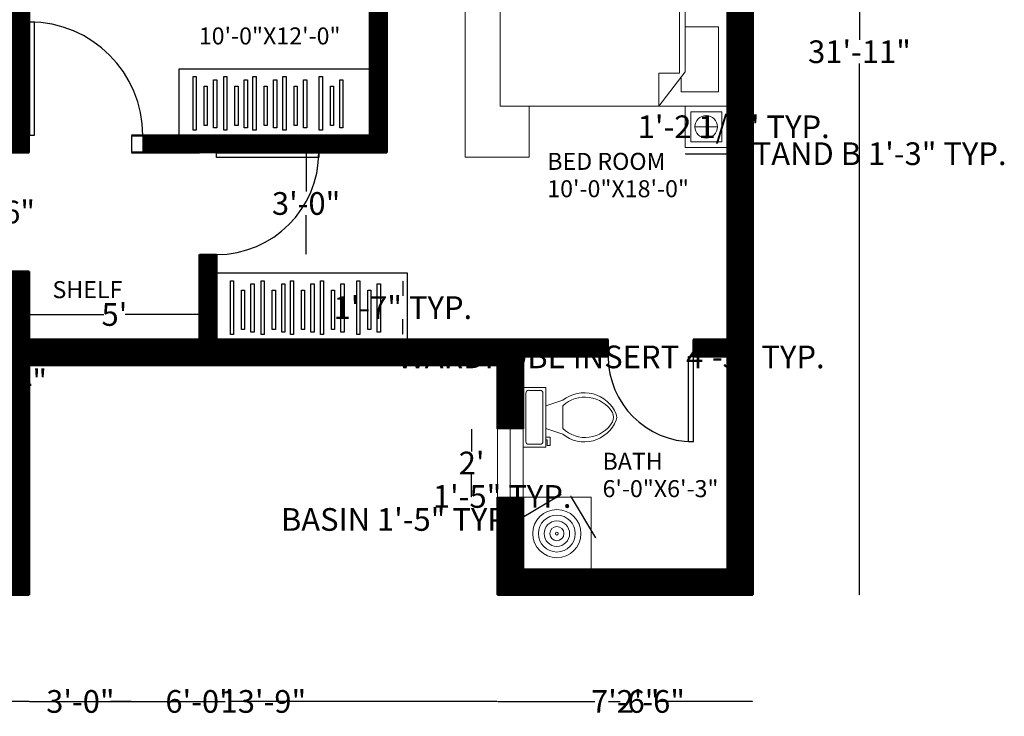
# Model space of a CAD drawing. Units: inches. Extents: x 348 to 1197, y 2602 to 3078.
# Tile 3 of 4: x 850 to 1197, y 2602 to 2848. Entities that reach past the tile are written whole.
import ezdxf

# ---------------------------------------------------------------- set-up
doc = ezdxf.new("R2010")
doc.units = ezdxf.units.IN
doc.header["$MEASUREMENT"] = 0
for name, color, linetype, lineweight in [('A-ANNO-DIMS', 20, 'Continuous', 18), ('A-ANNO-TEXT', 104, 'Continuous', 18), ('A-AREA-IDEN', 104, 'Continuous', 18), ('A-FLOR-CASE', 5, 'Continuous', 25), ('A-FLOR-FIXT', 9, 'Continuous', 18), ('A-WALL-PATT', 250, 'Continuous', 13), ('bed', 5, 'Continuous', 18), ('doors', 1, 'Continuous', 25), ('walls', 4, 'Continuous', 50), ('windows', 2, 'Continuous', 18)]:
    doc.layers.add(name, color=color, linetype=linetype, lineweight=lineweight)
doc.styles.get("Standard").update_dxf_attribs({"font": 'arial.ttf'})
doc.dimstyles.get("Standard").update_dxf_attribs({"dimtxt": 8, "dimasz": 0.18, "dimexe": 0.18, "dimexo": 0.0625, "dimgap": 0.09, "dimtad": 0, "dimtih": 1, "dimtoh": 1, "dimdec": 0, "dimzin": 0, "dimdsep": 46, "dimlunit": 3, "dimtxsty": 'Standard', "dimblk": 'DOT', "dimcen": 0.09, "dimse1": 1, "dimse2": 1, "dimadec": 0, "dimazin": 0, "dimtfac": 1, "dimtdec": 0, "dimtofl": 0, "dimtmove": 0, "dimatfit": 3, "dimfxl": 1, "dimtolj": 1, "dimtzin": 0, "dimarcsym": 0})

# ---------------------------------------------------------------- blocks, each defined once
blk = doc.blocks.new('*U4')
for p, q in [((0, 0), (0, -6)), ((40, 0), (40, -6))]:
    blk.add_line(p, q)
blk.add_lwpolyline([(0, 0), (0, 40), (1.75, 40), (1.75, 0)], close=True)
blk.add_arc((0, 0), 40, 0, 90)
blk = doc.blocks.new('*U5')
for p, q in [((-30, 0), (-30, 6)), ((0, 0), (0, 6))]:
    blk.add_line(p, q)
blk.add_lwpolyline([(0, 0), (0, -30), (-1.75, -30), (-1.75, 0)], close=True)
blk.add_arc((0, 0), 30, 180, 270)
blk = doc.blocks.new('*U7')
for p, q in [((0, 0), (0, -6)), ((36, 0), (36, -6))]:
    blk.add_line(p, q)
blk.add_lwpolyline([(0, 0), (0, 36), (1.75, 36), (1.75, 0)], close=True)
blk.add_arc((0, 0), 36, 360, 90)
blk = doc.blocks.new('*U13')
for p, q in [((5.98, 9.51), (1.98, 9.5)), ((7.99, 4.02), (13.99, 6.03)), ((13.99, 4.03), (14.01, -3.97)), ((8.01, -3.98), (14.01, -5.97)), ((8.01, -6.98), (9.51, -6.98)), ((8.52, -7.98), (8.02, -7.98)), ((8.52, -9.98), (8.52, -7.98)), ((9.52, -9.98), (8.52, -9.98)), ((9.51, -6.98), (9.52, -9.98))]:
    blk.add_line(p, q)
blk.add_lwpolyline([(7.98, 10.51), (-0.02, 10.5), (0.02, -10.5), (8.02, -10.48)], close=True)
for points in [[(0.98, 8.5), (1.02, -8.5)], [(7.02, -8.49), (6.98, 8.51)], [(2.02, -9.5), (6.02, -9.49)]]:
    blk.add_lwpolyline(points)
for centre, radius, start, end in [((1.86, 8.63), 0.884, 81.9774, 188.2376), ((6.11, 8.64), 0.884, 351.9774, 98.2376), ((21.59, -3.48), 12.17, 22.136, 128.6382), ((21.83, -4.16), 11.33, 31.1605, 133.7396), ((27.88, 0.05), 4, 335.8394, 24.3757), ((29, 0.05), 4, 344.9681, 15.247), ((21.57, 3.56), 12.17, 231.5766, 338.079), ((21.81, 4.24), 11.33, 226.4753, 329.0544), ((1.89, -8.62), 0.884, 171.9774, 278.2376), ((6.14, -8.61), 0.884, 261.9774, 8.2376)]:
    blk.add_arc(centre, radius, start, end)
blk = doc.blocks.new('_Dot')
at = {"color": 0, "linetype": 'ByBlock', "lineweight": -2}
blk.add_line((-0.5, 0), (-1, 0), dxfattribs=at)
at = {"color": 0, "linetype": 'ByBlock', "const_width": 0.5}
blk.add_lwpolyline([(-0.25, 0, 1), (0.25, 0, 1)], format="xyb", close=True, dxfattribs=at)
blk = doc.blocks.new('*D26')
at = {"layer": 'A-ANNO-DIMS', "color": 0, "lineweight": -2, "transparency": 16777216}
for p, q in [((843.28, 2801.02), (843.28, 2784.38)), ((843.28, 2759.38), (843.28, 2776.03))]:
    blk.add_line(p, q, dxfattribs=at)
at = {"layer": 'Defpoints', "color": 0, "transparency": 16777216}
for p in [(843.28, 2801.2), (843.28, 2759.2), (843.28, 2759.2)]:
    blk.add_point(p, dxfattribs=at)
at = {"layer": 'A-ANNO-DIMS', "color": 0, "lineweight": -2, "transparency": 16777216, "xscale": 0.18, "yscale": 0.18, "zscale": 0.18}
for p, rotation in [((843.28, 2801.2), 90), ((843.28, 2759.2), 270)]:
    blk.add_blockref('_Dot', p, dxfattribs=dict(at, rotation=rotation))
at = {"layer": 'A-ANNO-DIMS', "color": 0, "transparency": 16777216, "insert": (843.28, 2780.2), "char_height": 8, "attachment_point": 5}
blk.add_mtext('\\A1;3\'-6"', dxfattribs=at)
blk = doc.blocks.new('*D27')
at = {"layer": 'A-ANNO-DIMS', "color": 0, "lineweight": -2, "transparency": 16777216}
for p, q in [((853.5, 2744.07), (879.55, 2744.07)), ((913.14, 2744.07), (887.09, 2744.07))]:
    blk.add_line(p, q, dxfattribs=at)
at = {"layer": 'Defpoints', "color": 0, "transparency": 16777216}
for p in [(853.32, 2744.07), (853.32, 2744.07), (913.32, 2744.07)]:
    blk.add_point(p, dxfattribs=at)
at = {"layer": 'A-ANNO-DIMS', "color": 0, "lineweight": -2, "transparency": 16777216, "xscale": 0.18, "yscale": 0.18, "zscale": 0.18, "rotation": 180}
blk.add_blockref('_Dot', (853.32, 2744.07), dxfattribs=at)
at = {"layer": 'A-ANNO-DIMS', "color": 0, "lineweight": -2, "transparency": 16777216, "xscale": 0.18, "yscale": 0.18, "zscale": 0.18}
blk.add_blockref('_Dot', (913.32, 2744.07), dxfattribs=at)
at = {"layer": 'A-ANNO-DIMS', "color": 0, "transparency": 16777216, "insert": (883.32, 2744.07), "char_height": 8, "attachment_point": 5}
blk.add_mtext("\\A1;5'", dxfattribs=at)
blk = doc.blocks.new('*D40')
at = {"layer": 'A-ANNO-DIMS', "color": 0, "lineweight": -2, "transparency": 16777216}
for p, q in [((1009.19, 2703.52), (1009.19, 2695.81)), ((1009.19, 2679.88), (1009.19, 2687.6))]:
    blk.add_line(p, q, dxfattribs=at)
at = {"layer": 'Defpoints', "color": 0, "transparency": 16777216}
for p in [(1009.19, 2703.7), (1018.32, 2703.7), (1018.32, 2679.7)]:
    blk.add_point(p, dxfattribs=at)
at = {"layer": 'A-ANNO-DIMS', "color": 0, "lineweight": -2, "transparency": 16777216, "xscale": 0.18, "yscale": 0.18, "zscale": 0.18}
for p, rotation in [((1009.19, 2703.7), 90), ((1009.19, 2679.7), 270)]:
    blk.add_blockref('_Dot', p, dxfattribs=dict(at, rotation=rotation))
at = {"layer": 'A-ANNO-DIMS', "color": 0, "transparency": 16777216, "insert": (1009.19, 2691.7), "char_height": 8, "attachment_point": 5}
blk.add_mtext("\\A1;2'", dxfattribs=at)
blk = doc.blocks.new('BED-QUEEN')
for p, q in [((24, 96), (0, 96)), ((0, 96), (0, 0)), ((24, 78), (24, 96)), ((92.39, 78), (12.39, 78)), ((12.39, 78), (12.39, 18)), ((75.49, 78), (75.49, 29.69)), ((77.49, 78), (77.49, 30.16)), ((77.49, 30.16), (68.23, 18)), ((68.23, 29.62), (75.49, 29.69)), ((68.23, 18), (68.23, 29.62)), ((12.39, 18), (92.39, 18)), ((22.56, 18), (22.56, 0)), ((22.56, 0), (0, 0))]:
    blk.add_line(p, q)
for points in [[(77.49, 51.42), (89.26, 51.42), (89.26, 74.34), (77.49, 74.34)], [(76.09, 28.32), (76.09, 23.06), (89.26, 23.06), (89.26, 45.98), (77.49, 45.98)]]:
    blk.add_lwpolyline(points)
blk = doc.blocks.new('NIGHTSTAND-LAMP-B')
for p, q in [((7.45, 11.24), (7.45, 3.27)), ((11.44, 7.26), (3.46, 7.26))]:
    blk.add_line(p, q)
for points in [[(14.9, 0), (0, 0), (0, 14.51), (14.9, 14.51)], [(12.9, 2), (2, 2), (2, 12.51), (12.9, 12.51)]]:
    blk.add_lwpolyline(points, close=True)
blk.add_circle((7.45, 7.26), 3.99)
blk = doc.blocks.new('WARDROBE-HANGER-SET')
for points in [[(0, 18.89), (1.11, 18.89), (1.11, 0), (0, 0)], [(7.23, 17.78), (8.34, 17.78), (8.34, 0.83), (7.23, 0.83)], [(10.85, 18.89), (11.96, 18.89), (11.96, 0), (10.85, 0)], [(18.08, 17.78), (19.19, 17.78), (19.19, 0.83), (18.08, 0.83)], [(21.14, 18.89), (22.25, 18.89), (22.25, 0), (21.14, 0)], [(28.37, 17.78), (29.49, 17.78), (29.49, 0.83), (28.37, 0.83)], [(31.71, 18.89), (32.82, 18.89), (32.82, 0), (31.71, 0)], [(38.94, 17.78), (40.06, 17.78), (40.06, 0.83), (38.94, 0.83)], [(44.51, 18.89), (45.62, 18.89), (45.62, 0), (44.51, 0)], [(51.74, 17.78), (52.85, 17.78), (52.85, 0.83), (51.74, 0.83)], [(3.89, 15.56), (5.01, 15.56), (5.01, 1.67), (3.89, 1.67)], [(14.74, 15.56), (15.86, 15.56), (15.86, 1.67), (14.74, 1.67)], [(25.04, 15.56), (26.15, 15.56), (26.15, 1.67), (25.04, 1.67)], [(35.61, 15.56), (36.72, 15.56), (36.72, 1.67), (35.61, 1.67)], [(48.4, 15.56), (49.51, 15.56), (49.51, 1.67), (48.4, 1.67)]]:
    blk.add_lwpolyline(points, close=True)
blk = doc.blocks.new('BASIN-ROUND')
for radius in [8.49, 8.49, 8.49, 6.49, 4.49, 4.49, 2.49, 0.487]:
    blk.add_circle((8.49, 8.49), radius)
blk = doc.blocks.new('*D58')
at = {"layer": 'A-ANNO-DIMS', "color": 0, "lineweight": -2, "transparency": 16777216}
for p, q in [((1040.68, 2680.54), (1026.44, 2671.99)), ((1026.13, 2671.81), (1025.95, 2671.81)), ((1026.28, 2671.9), (1026.13, 2671.81))]:
    blk.add_line(p, q, dxfattribs=at)
at = {"layer": 'Defpoints', "color": 0, "transparency": 16777216}
for p in [(1042.15, 2678.45), (1026.28, 2671.9), (1027.59, 2669.72)]:
    blk.add_point(p, dxfattribs=at)
at = {"layer": 'A-ANNO-DIMS', "color": 0, "lineweight": -2, "transparency": 16777216, "xscale": 0.18, "yscale": 0.18, "zscale": 0.18}
for p, rotation in [((1040.84, 2680.63), 30.96375653207271), ((1026.28, 2671.9), 210.9637565320727)]:
    blk.add_blockref('_Dot', p, dxfattribs=dict(at, rotation=rotation))
at = {"layer": 'A-ANNO-DIMS', "color": 0, "transparency": 16777216, "insert": (983.33, 2671.81), "char_height": 8, "attachment_point": 5}
blk.add_mtext('\\A1;BASIN 1\'-5" TYP.', dxfattribs=at)
blk = doc.blocks.new('*D59')
at = {"layer": 'A-ANNO-DIMS', "color": 0, "lineweight": -2, "transparency": 16777216}
for p, q in [((1044.24, 2679.92), (1044.06, 2679.92)), ((1044.33, 2679.76), (1044.24, 2679.92)), ((1052.97, 2665.36), (1044.42, 2679.61))]:
    blk.add_line(p, q, dxfattribs=at)
at = {"layer": 'Defpoints', "color": 0, "transparency": 16777216}
for p in [(1044.33, 2679.76), (1042.15, 2678.45), (1050.88, 2663.9)]:
    blk.add_point(p, dxfattribs=at)
at = {"layer": 'A-ANNO-DIMS', "color": 0, "lineweight": -2, "transparency": 16777216, "xscale": 0.18, "yscale": 0.18, "zscale": 0.18}
for p, rotation in [((1044.33, 2679.76), 120.9637565320735), ((1053.06, 2665.21), 300.9637565320735)]:
    blk.add_blockref('_Dot', p, dxfattribs=dict(at, rotation=rotation))
at = {"layer": 'A-ANNO-DIMS', "color": 0, "transparency": 16777216, "insert": (1019.96, 2679.92), "char_height": 8, "attachment_point": 5}
blk.add_mtext('\\A1;1\'-5" TYP.', dxfattribs=at)
blk = doc.blocks.new('*D60')
at = {"layer": 'A-ANNO-DIMS', "color": 0, "lineweight": -2, "transparency": 16777216}
for p, q in [((924.36, 2729.12), (976.85, 2729.12)), ((977.03, 2729.12), (977.21, 2729.12))]:
    blk.add_line(p, q, dxfattribs=at)
at = {"layer": 'Defpoints', "color": 0, "transparency": 16777216}
for p in [(924.18, 2737.05), (977.03, 2737.05), (977.03, 2729.12)]:
    blk.add_point(p, dxfattribs=at)
at = {"layer": 'A-ANNO-DIMS', "color": 0, "lineweight": -2, "transparency": 16777216, "xscale": 0.18, "yscale": 0.18, "zscale": 0.18, "rotation": 180}
blk.add_blockref('_Dot', (924.18, 2729.12), dxfattribs=at)
at = {"layer": 'A-ANNO-DIMS', "color": 0, "lineweight": -2, "transparency": 16777216, "xscale": 0.18, "yscale": 0.18, "zscale": 0.18}
blk.add_blockref('_Dot', (977.03, 2729.12), dxfattribs=at)
at = {"layer": 'A-ANNO-DIMS', "color": 0, "transparency": 16777216, "insert": (1058.35, 2729.12), "char_height": 8, "attachment_point": 5}
blk.add_mtext('\\A1;WARDROBE INSERT 4\'-5" TYP.', dxfattribs=at)
blk = doc.blocks.new('*D61')
at = {"layer": 'A-ANNO-DIMS', "color": 0, "lineweight": -2, "transparency": 16777216}
for p, q in [((984.96, 2755.76), (984.96, 2750.6)), ((984.96, 2737.23), (984.96, 2742.38))]:
    blk.add_line(p, q, dxfattribs=at)
at = {"layer": 'Defpoints', "color": 0, "transparency": 16777216}
for p in [(977.03, 2755.94), (984.96, 2755.94), (977.03, 2737.05)]:
    blk.add_point(p, dxfattribs=at)
at = {"layer": 'A-ANNO-DIMS', "color": 0, "lineweight": -2, "transparency": 16777216, "xscale": 0.18, "yscale": 0.18, "zscale": 0.18}
for p, rotation in [((984.96, 2755.94), 90), ((984.96, 2737.05), 270)]:
    blk.add_blockref('_Dot', p, dxfattribs=dict(at, rotation=rotation))
at = {"layer": 'A-ANNO-DIMS', "color": 0, "transparency": 16777216, "insert": (984.96, 2746.49), "char_height": 8, "attachment_point": 5}
blk.add_mtext('\\A1;1\'-7" TYP.', dxfattribs=at)
blk = doc.blocks.new('*D66')
at = {"layer": 'A-ANNO-DIMS', "color": 0, "lineweight": -2, "transparency": 16777216}
for p, q in [((1084.6, 2800.75), (1099.14, 2800.75)), ((1099.32, 2800.75), (1099.5, 2800.75))]:
    blk.add_line(p, q, dxfattribs=at)
at = {"layer": 'Defpoints', "color": 0, "transparency": 16777216}
for p in [(1084.42, 2802.98), (1099.32, 2802.98), (1099.32, 2800.75)]:
    blk.add_point(p, dxfattribs=at)
at = {"layer": 'A-ANNO-DIMS', "color": 0, "lineweight": -2, "transparency": 16777216, "xscale": 0.18, "yscale": 0.18, "zscale": 0.18, "rotation": 180}
blk.add_blockref('_Dot', (1084.42, 2800.75), dxfattribs=at)
at = {"layer": 'A-ANNO-DIMS', "color": 0, "lineweight": -2, "transparency": 16777216, "xscale": 0.18, "yscale": 0.18, "zscale": 0.18}
blk.add_blockref('_Dot', (1099.32, 2800.75), dxfattribs=at)
at = {"layer": 'A-ANNO-DIMS', "color": 0, "transparency": 16777216, "insert": (1149.72, 2800.75), "char_height": 8, "attachment_point": 5}
blk.add_mtext('\\A1;STAND B 1\'-3" TYP.', dxfattribs=at)
blk = doc.blocks.new('*D67')
at = {"layer": 'A-ANNO-DIMS', "color": 0, "lineweight": -2, "transparency": 16777216}
for p, q in [((1101.55, 2817.32), (1101.55, 2814.47)), ((1101.55, 2803.16), (1101.55, 2806.01))]:
    blk.add_line(p, q, dxfattribs=at)
at = {"layer": 'Defpoints', "color": 0, "transparency": 16777216}
for p in [(1099.32, 2817.5), (1101.55, 2817.5), (1099.32, 2802.98)]:
    blk.add_point(p, dxfattribs=at)
at = {"layer": 'A-ANNO-DIMS', "color": 0, "lineweight": -2, "transparency": 16777216, "xscale": 0.18, "yscale": 0.18, "zscale": 0.18}
for p, rotation in [((1101.55, 2817.5), 90), ((1101.55, 2802.98), 270)]:
    blk.add_blockref('_Dot', p, dxfattribs=dict(at, rotation=rotation))
at = {"layer": 'A-ANNO-DIMS', "color": 0, "transparency": 16777216, "insert": (1101.55, 2810.24), "char_height": 8, "attachment_point": 5}
blk.add_mtext('\\A1;1\'-2 1/2" TYP.', dxfattribs=at)
blk = doc.blocks.new('*D69')
at = {"layer": 'A-ANNO-DIMS', "color": 0, "lineweight": -2, "transparency": 16777216}
for p, q in [((1145.87, 3028.02), (1145.87, 2840.88)), ((1145.87, 2645.38), (1145.87, 2832.53))]:
    blk.add_line(p, q, dxfattribs=at)
at = {"layer": 'Defpoints', "color": 0, "transparency": 16777216}
for p in [(1108.32, 3028.2), (1145.87, 3028.2), (1108.32, 2645.2)]:
    blk.add_point(p, dxfattribs=at)
at = {"layer": 'A-ANNO-DIMS', "color": 0, "lineweight": -2, "transparency": 16777216, "xscale": 0.18, "yscale": 0.18, "zscale": 0.18}
for p, rotation in [((1145.87, 3028.2), 90), ((1145.87, 2645.2), 270)]:
    blk.add_blockref('_Dot', p, dxfattribs=dict(at, rotation=rotation))
at = {"layer": 'A-ANNO-DIMS', "color": 0, "transparency": 16777216, "insert": (1145.87, 2836.7), "char_height": 8, "attachment_point": 5}
blk.add_mtext('\\A1;31\'-11"', dxfattribs=at)
blk = doc.blocks.new('*D72')
at = {"layer": 'A-ANNO-DIMS', "color": 0, "lineweight": -2, "transparency": 16777216}
for p, q in [((532.5, 2607.65), (678.92, 2607.65)), ((853.14, 2607.65), (706.72, 2607.65))]:
    blk.add_line(p, q, dxfattribs=at)
at = {"layer": 'Defpoints', "color": 0, "transparency": 16777216}
for p in [(532.32, 2645.2), (853.32, 2645.2), (853.32, 2607.65)]:
    blk.add_point(p, dxfattribs=at)
at = {"layer": 'A-ANNO-DIMS', "color": 0, "lineweight": -2, "transparency": 16777216, "xscale": 0.18, "yscale": 0.18, "zscale": 0.18, "rotation": 180}
blk.add_blockref('_Dot', (532.32, 2607.65), dxfattribs=at)
at = {"layer": 'A-ANNO-DIMS', "color": 0, "lineweight": -2, "transparency": 16777216, "xscale": 0.18, "yscale": 0.18, "zscale": 0.18}
blk.add_blockref('_Dot', (853.32, 2607.65), dxfattribs=at)
at = {"layer": 'A-ANNO-DIMS', "color": 0, "transparency": 16777216, "insert": (692.82, 2607.65), "char_height": 8, "attachment_point": 5}
blk.add_mtext('\\A1;26\'-9"', dxfattribs=at)
blk = doc.blocks.new('*D73')
at = {"layer": 'A-ANNO-DIMS', "color": 0, "lineweight": -2, "transparency": 16777216}
for p, q in [((853.5, 2607.65), (922.36, 2607.65)), ((1018.14, 2607.65), (949.27, 2607.65))]:
    blk.add_line(p, q, dxfattribs=at)
at = {"layer": 'Defpoints', "color": 0, "transparency": 16777216}
for p in [(853.32, 2645.2), (1018.32, 2645.2), (1018.32, 2607.65)]:
    blk.add_point(p, dxfattribs=at)
at = {"layer": 'A-ANNO-DIMS', "color": 0, "lineweight": -2, "transparency": 16777216, "xscale": 0.18, "yscale": 0.18, "zscale": 0.18, "rotation": 180}
blk.add_blockref('_Dot', (853.32, 2607.65), dxfattribs=at)
at = {"layer": 'A-ANNO-DIMS', "color": 0, "lineweight": -2, "transparency": 16777216, "xscale": 0.18, "yscale": 0.18, "zscale": 0.18}
blk.add_blockref('_Dot', (1018.32, 2607.65), dxfattribs=at)
at = {"layer": 'A-ANNO-DIMS', "color": 0, "transparency": 16777216, "insert": (935.82, 2607.65), "char_height": 8, "attachment_point": 5}
blk.add_mtext('\\A1;13\'-9"', dxfattribs=at)
blk = doc.blocks.new('*D74')
at = {"layer": 'A-ANNO-DIMS', "color": 0, "lineweight": -2, "transparency": 16777216}
for p, q in [((1018.5, 2607.65), (1052.63, 2607.65)), ((1108.14, 2607.65), (1074.01, 2607.65))]:
    blk.add_line(p, q, dxfattribs=at)
at = {"layer": 'Defpoints', "color": 0, "transparency": 16777216}
for p in [(1018.32, 2645.2), (1108.32, 2645.2), (1108.32, 2607.65)]:
    blk.add_point(p, dxfattribs=at)
at = {"layer": 'A-ANNO-DIMS', "color": 0, "lineweight": -2, "transparency": 16777216, "xscale": 0.18, "yscale": 0.18, "zscale": 0.18, "rotation": 180}
blk.add_blockref('_Dot', (1018.32, 2607.65), dxfattribs=at)
at = {"layer": 'A-ANNO-DIMS', "color": 0, "lineweight": -2, "transparency": 16777216, "xscale": 0.18, "yscale": 0.18, "zscale": 0.18}
blk.add_blockref('_Dot', (1108.32, 2607.65), dxfattribs=at)
at = {"layer": 'A-ANNO-DIMS', "color": 0, "transparency": 16777216, "insert": (1063.32, 2607.65), "char_height": 8, "attachment_point": 5}
blk.add_mtext('\\A1;7\'-6"', dxfattribs=at)
blk = doc.blocks.new('*D78')
at = {"layer": 'A-ANNO-DIMS', "color": 0, "lineweight": -2, "transparency": 16777216}
for p, q in [((853.5, 2607.65), (860.6, 2607.65)), ((889.14, 2607.65), (882.04, 2607.65))]:
    blk.add_line(p, q, dxfattribs=at)
at = {"layer": 'Defpoints', "color": 0, "transparency": 16777216}
for p in [(853.32, 2807.2), (889.32, 2807.2), (889.32, 2607.65)]:
    blk.add_point(p, dxfattribs=at)
at = {"layer": 'A-ANNO-DIMS', "color": 0, "lineweight": -2, "transparency": 16777216, "xscale": 0.18, "yscale": 0.18, "zscale": 0.18, "rotation": 180}
blk.add_blockref('_Dot', (853.32, 2607.65), dxfattribs=at)
at = {"layer": 'A-ANNO-DIMS', "color": 0, "lineweight": -2, "transparency": 16777216, "xscale": 0.18, "yscale": 0.18, "zscale": 0.18}
blk.add_blockref('_Dot', (889.32, 2607.65), dxfattribs=at)
at = {"layer": 'A-ANNO-DIMS', "color": 0, "transparency": 16777216, "insert": (871.32, 2607.65), "char_height": 8, "attachment_point": 5}
blk.add_mtext('\\A1;3\'-0"', dxfattribs=at)
blk = doc.blocks.new('*D79')
at = {"layer": 'A-ANNO-DIMS', "color": 0, "lineweight": -2, "transparency": 16777216}
for p, q in [((950.87, 2801.02), (950.87, 2787.38)), ((950.87, 2765.38), (950.87, 2779.03))]:
    blk.add_line(p, q, dxfattribs=at)
at = {"layer": 'Defpoints', "color": 0, "transparency": 16777216}
for p in [(913.32, 2801.2), (913.32, 2765.2), (950.87, 2765.2)]:
    blk.add_point(p, dxfattribs=at)
at = {"layer": 'A-ANNO-DIMS', "color": 0, "lineweight": -2, "transparency": 16777216, "xscale": 0.18, "yscale": 0.18, "zscale": 0.18}
for p, rotation in [((950.87, 2801.2), 90), ((950.87, 2765.2), 270)]:
    blk.add_blockref('_Dot', p, dxfattribs=dict(at, rotation=rotation))
at = {"layer": 'A-ANNO-DIMS', "color": 0, "transparency": 16777216, "insert": (950.87, 2783.2), "char_height": 8, "attachment_point": 5}
blk.add_mtext('\\A1;3\'-0"', dxfattribs=at)
blk = doc.blocks.new('*D80')
at = {"layer": 'A-ANNO-DIMS', "color": 0, "lineweight": -2, "transparency": 16777216}
for p, q in [((1057.5, 2607.65), (1061.53, 2607.65)), ((1087.14, 2607.65), (1083.11, 2607.65))]:
    blk.add_line(p, q, dxfattribs=at)
at = {"layer": 'Defpoints', "color": 0, "transparency": 16777216}
for p in [(1057.32, 2735.2), (1087.32, 2735.2), (1087.32, 2607.65)]:
    blk.add_point(p, dxfattribs=at)
at = {"layer": 'A-ANNO-DIMS', "color": 0, "lineweight": -2, "transparency": 16777216, "xscale": 0.18, "yscale": 0.18, "zscale": 0.18, "rotation": 180}
blk.add_blockref('_Dot', (1057.32, 2607.65), dxfattribs=at)
at = {"layer": 'A-ANNO-DIMS', "color": 0, "lineweight": -2, "transparency": 16777216, "xscale": 0.18, "yscale": 0.18, "zscale": 0.18}
blk.add_blockref('_Dot', (1087.32, 2607.65), dxfattribs=at)
at = {"layer": 'A-ANNO-DIMS', "color": 0, "transparency": 16777216, "insert": (1072.32, 2607.65), "char_height": 8, "attachment_point": 5}
blk.add_mtext('\\A1;2\'-6"', dxfattribs=at)
blk = doc.blocks.new('*D81')
at = {"layer": 'A-ANNO-DIMS', "color": 0, "lineweight": -2, "transparency": 16777216}
for p, q in [((877.5, 2607.65), (902.57, 2607.65)), ((949.14, 2607.65), (924.06, 2607.65))]:
    blk.add_line(p, q, dxfattribs=at)
at = {"layer": 'Defpoints', "color": 0, "transparency": 16777216}
for p in [(877.32, 2951.2), (949.32, 2951.2), (949.32, 2607.65)]:
    blk.add_point(p, dxfattribs=at)
at = {"layer": 'A-ANNO-DIMS', "color": 0, "lineweight": -2, "transparency": 16777216, "xscale": 0.18, "yscale": 0.18, "zscale": 0.18, "rotation": 180}
blk.add_blockref('_Dot', (877.32, 2607.65), dxfattribs=at)
at = {"layer": 'A-ANNO-DIMS', "color": 0, "lineweight": -2, "transparency": 16777216, "xscale": 0.18, "yscale": 0.18, "zscale": 0.18}
blk.add_blockref('_Dot', (949.32, 2607.65), dxfattribs=at)
at = {"layer": 'A-ANNO-DIMS', "color": 0, "transparency": 16777216, "insert": (913.32, 2607.65), "char_height": 8, "attachment_point": 5}
blk.add_mtext('\\A1;6\'-0"', dxfattribs=at)
blk = doc.blocks.new('*D83')
at = {"layer": 'A-ANNO-DIMS', "color": 0, "lineweight": -2, "transparency": 16777216}
for p, q in [((829.5, 2720.69), (829.32, 2720.69)), ((829.32, 2720.69), (829.32, 2711.27)), ((829.23, 2695.09), (829.41, 2695.09)), ((829.32, 2695), (829.32, 2695.18))]:
    blk.add_line(p, q, dxfattribs=at)
at = {"layer": 'Defpoints', "color": 0, "transparency": 16777216}
for p in [(829.32, 2711.09), (829.32, 2695.09)]:
    blk.add_point(p, dxfattribs=at)
at = {"layer": 'A-ANNO-DIMS', "color": 0, "lineweight": -2, "transparency": 16777216, "xscale": 0.18, "yscale": 0.18, "zscale": 0.18, "rotation": 269.9894074428831}
blk.add_blockref('_Dot', (829.32, 2711.09), dxfattribs=at)
at = {"layer": 'A-ANNO-DIMS', "color": 0, "transparency": 16777216, "insert": (844.05, 2720.69), "char_height": 8, "attachment_point": 5}
blk.add_mtext('\\A1;R1\'-4"', dxfattribs=at)

msp = doc.modelspace()

# ---------------------------------------------------------------- hatches: boundary and pattern name
at = {"layer": 'A-WALL-PATT'}
h = msp.add_hatch(dxfattribs=at)
h.set_pattern_fill('ANSI31', color=256, scale=1.5)
h.paths.add_polyline_path([(481.32, 2951.2), (509.32, 2951.2), (509.32, 2960.2), (505.32, 2960.2), (481.32, 2960.2), (481.32, 3018.2), (452.32, 3018.2), (452.32, 3009.2), (472.32, 3009.2), (472.32, 2943.2), (481.32, 2943.2)], flags=17)
h.paths.add_polyline_path([(428.32, 3018.2), (399.32, 3018.2), (399.32, 2904.2), (472.32, 2904.2), (472.32, 2726.2), (532.32, 2726.2), (532.32, 2696.2), (541.32, 2696.2), (541.32, 2726.2), (565.32, 2726.2), (565.32, 2735.2), (481.32, 2735.2), (481.32, 2758.72), (481.32, 2809.83), (481.31, 2809.83), (481.31, 2824.34), (481.31, 2884.34), (481.31, 2884.34), (481.31, 2898.86), (481.32, 2913.2), (472.32, 2913.2), (408.32, 2913.2), (408.32, 3009.2), (428.32, 3009.2)])
h.paths.add_polyline_path([(796.32, 2654.2), (769.32, 2654.2), (769.32, 2753.2), (769.32, 2759.2), (763.32, 2759.2), (763.32, 2735.2), (763.32, 2654.2), (541.32, 2654.2), (532.32, 2654.2), (532.32, 2645.2), (796.32, 2645.2)])
h.paths.add_polyline_path([(853.32, 2726.2), (1018.32, 2726.2), (1018.32, 2703.7), (1027.32, 2703.7), (1027.32, 2729.2), (1057.32, 2729.2), (1057.32, 2735.2), (919.32, 2735.2), (919.32, 2758.72), (919.32, 2765.2), (913.32, 2765.2), (913.32, 2735.2), (853.32, 2735.2), (853.32, 2759.2), (799.32, 2759.2), (799.32, 2753.2), (847.32, 2753.2), (847.32, 2654.2), (820.32, 2654.2), (820.32, 2645.2), (853.32, 2645.2)])
h.paths.add_polyline_path([(640.32, 2960.2), (577.32, 2960.2), (577.32, 2951.2), (601.32, 2951.2), (601.32, 2735.2), (601.32, 2726.2), (607.32, 2726.2), (607.32, 2951.2), (640.32, 2951.2)])
h.paths.add_polyline_path([(877.32, 2960.2), (688.32, 2960.2), (688.32, 2951.2), (745.32, 2951.2), (745.32, 2837.2), (751.32, 2837.2), (751.32, 2951.2), (847.32, 2951.2), (847.32, 2807.2), (751.32, 2807.2), (745.32, 2807.2), (745.32, 2801.2), (853.32, 2801.2), (853.32, 2807.2), (853.32, 2951.2), (877.32, 2951.2)])
h.paths.add_polyline_path([(1003.32, 2960.2), (949.32, 2960.2), (949.32, 2951.2), (973.32, 2951.2), (973.32, 2807.2), (906.15, 2807.2), (893.32, 2807.2), (893.32, 2801.2), (913.32, 2801.2), (919.32, 2801.2), (955.32, 2801.2), (979.32, 2801.2), (979.32, 2951.2), (1003.32, 2951.2)])
h.paths.add_polyline_path([(1108.32, 2960.2), (1104.32, 2960.2), (1075.32, 2960.2), (1075.32, 2951.2), (1099.32, 2951.2), (1099.32, 2735.2), (1087.32, 2735.2), (1087.32, 2729.2), (1099.32, 2729.2), (1099.32, 2654.2), (1027.32, 2654.2), (1027.32, 2679.7), (1018.32, 2679.7), (1018.32, 2645.2), (1108.32, 2645.2)])
h.paths.add_polyline_path([(509.32, 2992.2), (505.32, 2992.2), (505.32, 2965.1), (509.32, 2965.1)], flags=16)
h.paths.add_polyline_path([(509.32, 3023.27), (505.32, 3023.27), (505.32, 2997.1), (509.32, 2997.1)])
h.paths.add_polyline_path([(576.46, 3028.2), (509.32, 3028.2), (509.32, 3024.2), (576.46, 3024.2)])
h.paths.add_polyline_path([(624.46, 3028.2), (581.36, 3028.2), (581.36, 3024.2), (624.46, 3024.2)])
h.paths.add_polyline_path([(672.46, 3028.2), (629.36, 3028.2), (629.36, 3024.2), (672.46, 3024.2)])
h.paths.add_polyline_path([(720.46, 3028.2), (677.36, 3028.2), (677.36, 3024.2), (720.46, 3024.2)])
h.paths.add_polyline_path([(768.46, 3028.2), (725.36, 3028.2), (725.36, 3024.2), (768.46, 3024.2)])
h.paths.add_polyline_path([(804.46, 3028.2), (773.36, 3028.2), (773.36, 3024.2), (804.46, 3024.2)])
h.paths.add_polyline_path([(852.46, 3028.2), (809.36, 3028.2), (809.36, 3024.2), (852.46, 3024.2)])
h.paths.add_polyline_path([(900.46, 3028.2), (857.36, 3028.2), (857.36, 3024.2), (900.46, 3024.2)])
h.paths.add_polyline_path([(948.46, 3028.2), (905.36, 3028.2), (905.36, 3024.2), (948.46, 3024.2)])
h.paths.add_polyline_path([(996.46, 3028.2), (953.36, 3028.2), (953.36, 3024.2), (996.46, 3024.2)])
h.paths.add_polyline_path([(1056.46, 3028.2), (1001.36, 3028.2), (1001.36, 3024.2), (1056.46, 3024.2)])
h.paths.add_polyline_path([(1103.42, 3028.2), (1061.36, 3028.2), (1061.36, 3024.2), (1103.42, 3024.2)])
h.paths.add_polyline_path([(1108.32, 3024.17), (1104.32, 3024.17), (1104.32, 2994.89), (1108.32, 2994.89)])
h.paths.add_polyline_path([(1108.32, 2989.99), (1104.32, 2989.99), (1104.32, 2965.1), (1108.32, 2965.1)])

# ---------------------------------------------------------------- linework, layer by layer
at = {"layer": 'A-FLOR-CASE'}
for points in [[(906.15, 2830.72), (973.32, 2830.72), (973.32, 2807.2), (906.15, 2807.2)], [(919.32, 2758.72), (986.49, 2758.72), (986.49, 2735.2), (919.32, 2735.2)]]:
    msp.add_lwpolyline(points, close=True, dxfattribs=at)
at = {"layer": 'A-FLOR-FIXT'}
for p, q in [((1027.32, 2679.7), (1051.32, 2679.7)), ((1051.32, 2679.7), (1051.32, 2654.2))]:
    msp.add_line(p, q, dxfattribs=at)
at = {"layer": 'doors'}
for p, q in [((853.32, 2807.2), (853.32, 2801.2)), ((889.32, 2807.2), (889.32, 2801.2)), ((913.32, 2801.2), (919.32, 2801.2)), ((913.32, 2765.2), (919.32, 2765.2)), ((1057.32, 2735.2), (1057.32, 2729.2)), ((1087.32, 2735.2), (1087.32, 2729.2))]:
    msp.add_line(p, q, dxfattribs=at)
at = {"layer": 'walls'}
for p, q in [((1108.32, 2960.2), (1108.32, 2645.2)), ((853.32, 2951.2), (853.32, 2807.2)), ((973.32, 2951.2), (973.32, 2807.2)), ((979.32, 2951.2), (979.32, 2801.2)), ((1099.32, 2951.2), (1099.32, 2735.2)), ((889.32, 2807.2), (973.32, 2807.2)), ((745.32, 2801.2), (853.32, 2801.2)), ((889.32, 2801.2), (913.32, 2801.2)), ((919.32, 2801.2), (979.32, 2801.2)), ((913.32, 2735.2), (913.32, 2765.2)), ((919.32, 2735.2), (919.32, 2765.2)), ((799.32, 2759.2), (853.32, 2759.2)), ((853.32, 2735.2), (853.32, 2759.2)), ((853.32, 2735.2), (913.32, 2735.2)), ((853.32, 2735.2), (913.32, 2735.2)), ((919.32, 2735.2), (1057.32, 2735.2)), ((1087.32, 2735.2), (1099.32, 2735.2)), ((1027.32, 2729.2), (1057.32, 2729.2)), ((1027.32, 2729.2), (1027.32, 2703.7)), ((1087.32, 2729.2), (1099.32, 2729.2)), ((1099.32, 2729.2), (1099.32, 2654.2)), ((853.32, 2726.2), (1018.32, 2726.2)), ((853.32, 2726.2), (853.32, 2645.2)), ((1018.32, 2726.2), (1018.32, 2703.7)), ((1018.32, 2679.7), (1018.32, 2645.2)), ((1027.32, 2679.7), (1027.32, 2654.2)), ((1027.32, 2654.2), (1099.32, 2654.2)), ((820.32, 2645.2), (853.32, 2645.2)), ((1018.32, 2645.2), (1108.32, 2645.2))]:
    msp.add_line(p, q, dxfattribs=at)
at = {"layer": 'windows'}
for p, q in [((1027.32, 2703.7), (1018.32, 2703.7)), ((1018.32, 2679.7), (1018.32, 2703.7)), ((1022.82, 2679.7), (1022.82, 2703.7)), ((1027.32, 2703.7), (1027.32, 2679.7)), ((1027.32, 2679.7), (1018.32, 2679.7))]:
    msp.add_line(p, q, dxfattribs=at)

# ---------------------------------------------------------------- block references
at = {"layer": 'A-FLOR-CASE'}
for p in [(911.01, 2809.05), (924.18, 2737.05)]:
    msp.add_blockref('WARDROBE-HANGER-SET', p, dxfattribs=at)
at = {"layer": 'A-FLOR-FIXT'}
for name, p, rotation in [('*U13', (1027.32, 2707.83), 359.8924611627634), ('BASIN-ROUND', (1050.88, 2663.9), 120.9637565320735)]:
    msp.add_blockref(name, p, dxfattribs=dict(at, rotation=rotation))
at = {"layer": 'bed'}
for name, p in [('BED-QUEEN', (1006.92, 2799.49)), ('NIGHTSTAND-LAMP-B', (1084.41, 2802.98))]:
    msp.add_blockref(name, p, dxfattribs=at)
at = {"layer": 'doors'}
for name, p in [('*U4', (853.32, 2807.2)), ('*U5', (1087.32, 2729.2))]:
    msp.add_blockref(name, p, dxfattribs=at)
at = {"layer": 'doors', "rotation": 270}
msp.add_blockref('*U7', (919.32, 2801.2), dxfattribs=at)

# ---------------------------------------------------------------- texts
at = {"layer": 'A-ANNO-TEXT'}
msp.add_text('SHELF', height=6, dxfattribs=at).set_placement((861.49, 2749.83))
at = {"layer": 'A-AREA-IDEN'}
for s, p in [('10\'-0"X12\'-0"', (913.05, 2839.27)), ('BED ROOM ', (1035.84, 2795.05)), ('10\'-0"X18\'-0"', (1035.84, 2785.41)), ('BATH ', (1055.32, 2689.31)), ('6\'-0"X6\'-3"', (1055.32, 2679.67))]:
    msp.add_text(s, height=6, dxfattribs=at).set_placement(p)

# ---------------------------------------------------------------- dimensions: what is measured, and where the dimension line sits
at = {"layer": 'A-ANNO-DIMS'}
for base, p1, p2, angle, override, picture, middle in [((1145.87, 3028.2), (1108.32, 2645.2), (1108.32, 3028.2), 90, {"dimdec": 1, "dimlfac": 1, "dimrnd": 0, "dimzin": 1, "dimdsep": 46, "dimlunit": 4, "dimfrac": 2}, '*D69', (1145.87, 2836.7)), ((843.28, 2759.2), (843.28, 2801.2), (843.28, 2759.2), 90, {"dimclrd": 0, "dimclre": 0, "dimclrt": 0}, '*D26', (843.28, 2780.2)), ((950.87, 2765.2), (913.32, 2801.2), (913.32, 2765.2), 270, {"dimdec": 1, "dimlfac": 1, "dimrnd": 0, "dimzin": 1, "dimdsep": 46, "dimlunit": 4, "dimfrac": 2}, '*D79', (950.87, 2783.2)), ((1009.19, 2703.7), (1018.32, 2679.7), (1018.32, 2703.7), 90, {"dimclrd": 0, "dimclre": 0, "dimclrt": 0}, '*D40', (1009.19, 2691.7))]:
    dim = msp.add_linear_dim(base=base, p1=p1, p2=p2, angle=angle, dimstyle='Standard', override=override, dxfattribs=at)
    dim.commit()
    dim.dimension.update_dxf_attribs({"geometry": picture, "text_midpoint": middle})
for base, p1, p2, override, picture, middle in [((949.32, 2607.65), (877.32, 2951.2), (949.32, 2951.2), {"dimdec": 1, "dimlfac": 1, "dimrnd": 0, "dimzin": 1, "dimdsep": 46, "dimlunit": 4, "dimfrac": 2}, '*D81', (913.32, 2607.65)), ((889.32, 2607.65), (853.32, 2807.2), (889.32, 2807.2), {"dimdec": 1, "dimlfac": 1, "dimrnd": 0, "dimzin": 1, "dimdsep": 46, "dimlunit": 4, "dimfrac": 2}, '*D78', (871.32, 2607.65)), ((853.32, 2744.07), (913.32, 2744.07), (853.32, 2744.07), {"dimclrd": 0, "dimclre": 0, "dimclrt": 0}, '*D27', (883.32, 2744.07)), ((1087.32, 2607.65), (1057.32, 2735.2), (1087.32, 2735.2), {"dimdec": 1, "dimlfac": 1, "dimrnd": 0, "dimzin": 1, "dimdsep": 46, "dimlunit": 4, "dimfrac": 2}, '*D80', (1072.32, 2607.65)), ((853.32, 2607.65), (532.32, 2645.2), (853.32, 2645.2), {"dimdec": 1, "dimlfac": 1, "dimrnd": 0, "dimzin": 1, "dimdsep": 46, "dimlunit": 4, "dimfrac": 2}, '*D72', (692.82, 2607.65)), ((1018.32, 2607.65), (853.32, 2645.2), (1018.32, 2645.2), {"dimdec": 1, "dimlfac": 1, "dimrnd": 0, "dimzin": 1, "dimdsep": 46, "dimlunit": 4, "dimfrac": 2}, '*D73', (935.82, 2607.65)), ((1108.32, 2607.65), (1018.32, 2645.2), (1108.32, 2645.2), {"dimdec": 1, "dimlfac": 1, "dimrnd": 0, "dimzin": 1, "dimdsep": 46, "dimlunit": 4, "dimfrac": 2}, '*D74', (1063.32, 2607.65))]:
    dim = msp.add_linear_dim(base=base, p1=p1, p2=p2, dimstyle='Standard', override=override, dxfattribs=at)
    dim.commit()
    dim.dimension.update_dxf_attribs({"geometry": picture, "text_midpoint": middle})
for base, p1, p2, angle, text, picture, middle in [((1101.55, 2817.5), (1099.32, 2802.98), (1099.32, 2817.5), 90, '<> TYP.', '*D67', (1101.55, 2810.24)), ((984.96, 2755.94), (977.03, 2737.05), (977.03, 2755.94), 90, '<> TYP.', '*D61', (984.96, 2746.49)), ((1026.28, 2671.9), (1042.15, 2678.45), (1027.59, 2669.72), 210.9638, 'BASIN <> TYP.', '*D58', (983.33, 2671.81)), ((1044.33, 2679.76), (1050.88, 2663.9), (1042.15, 2678.45), 120.9638, '<> TYP.', '*D59', (1019.96, 2679.92))]:
    dim = msp.add_linear_dim(base=base, p1=p1, p2=p2, angle=angle, text=text, dimstyle='Standard', override={"dimdec": 1, "dimlfac": 1, "dimrnd": 0, "dimzin": 1, "dimdsep": 46, "dimlunit": 4, "dimfrac": 2}, dxfattribs=at)
    dim.commit()
    dim.dimension.update_dxf_attribs({"geometry": picture, "text_midpoint": middle})
for base, p1, p2, text, picture, middle in [((1099.32, 2800.75), (1084.42, 2802.98), (1099.32, 2802.98), 'STAND B <> TYP.', '*D66', (1149.72, 2800.75)), ((977.0278, 2729.1202), (924.176, 2737.048), (977.0278, 2737.048), 'WARDROBE INSERT <> TYP.', '*D60', (1058.3483, 2729.1202))]:
    dim = msp.add_linear_dim(base=base, p1=p1, p2=p2, text=text, dimstyle='Standard', override={"dimdec": 1, "dimlfac": 1, "dimrnd": 0, "dimzin": 1, "dimdsep": 46, "dimlunit": 4, "dimfrac": 2}, dxfattribs=at)
    dim.commit()
    dim.dimension.update_dxf_attribs({"geometry": picture, "text_midpoint": middle})
dim = msp.add_radius_dim(center=(829.32, 2695.09), mpoint=(829.32, 2711.09), dimstyle='Standard', override={"dimdec": 1, "dimlfac": 1, "dimrnd": 0, "dimzin": 1, "dimdsep": 46, "dimlunit": 4, "dimfrac": 2}, dxfattribs=at)
dim.commit()
dim.dimension.update_dxf_attribs({"geometry": '*D83', "text_midpoint": (844.05, 2720.69), "dimtype": 164})

doc.saveas('drawing.dxf')
